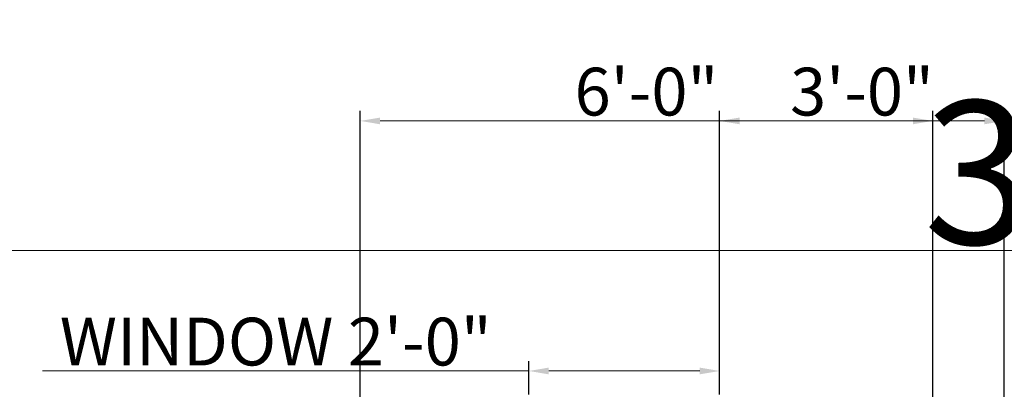
# Model space of a CAD drawing. Units: inches. Extents: x 2696 to 3240, y 1564 to 2310.
# Tile 63 of 76: x 2842 to 2966, y 2264 to 2310. Entities that reach past the tile are written whole.
import ezdxf

# ---------------------------------------------------------------- set-up
doc = ezdxf.new("R2010")
doc.units = ezdxf.units.IN
doc.layers.add('A-ANNO-DIMS', color=3, linetype='Continuous', lineweight=18)
doc.styles.add('TIMES NEW', font='times.ttf')
doc.dimstyles.new('Siddhuu', dxfattribs={"dimtxt": 6, "dimasz": 2.5, "dimexe": 1.25, "dimexo": 0.625, "dimtad": 1, "dimdec": 1, "dimlunit": 4, "dimtxsty": 'TIMES NEW', "dimcen": 2.5, "dimclrd": 256, "dimclre": 1, "dimclrt": 7, "dimadec": 0, "dimazin": 0, "dimtfac": 1, "dimtdec": 1, "dimtmove": 0, "dimatfit": 3, "dimfxl": 1, "dimtolj": 1, "dimlwd": -1, "dimarcsym": 0})

# ---------------------------------------------------------------- blocks, each defined once
blk = doc.blocks.new('*D9')
at = {"layer": 'A-ANNO-DIMS', "color": 0, "lineweight": -2, "transparency": 16777216}
for p, q in [((2745.61, 2262.83), (2745.61, 2282.19)), ((3199.61, 2262.83), (3199.61, 2282.19))]:
    blk.add_line(p, q, dxfattribs=at)
at = {"layer": 'A-ANNO-DIMS', "color": 0, "transparency": 16777216}
blk.add_line((2757.61, 2280.94), (3187.61, 2280.94), dxfattribs=at)
for points in [[(2757.61, 2282.94), (2757.61, 2278.94), (2745.61, 2280.94)], [(3187.61, 2282.94), (3187.61, 2278.94), (3199.61, 2280.94)]]:
    blk.add_solid(points, dxfattribs=at)
at = {"layer": 'Defpoints', "color": 0, "transparency": 16777216}
for p in [(3199.61, 2280.94), (2745.61, 2262.2), (3199.61, 2262.2)]:
    blk.add_point(p, dxfattribs=at)
at = {"layer": 'A-ANNO-DIMS', "color": 0, "transparency": 16777216, "insert": (2972.61, 2290.72), "char_height": 18, "attachment_point": 5, "style": 'TIMES NEW'}
blk.add_mtext("\\A1;36'", dxfattribs=at)
blk = doc.blocks.new('*D20')
at = {"layer": 'A-ANNO-DIMS', "color": 1, "lineweight": -2, "transparency": 16777216}
for p, q in [((2905.91, 2262.83), (2905.91, 2267.05)), ((2929.91, 2262.83), (2929.91, 2267.05))]:
    blk.add_line(p, q, dxfattribs=at)
at = {"layer": 'A-ANNO-DIMS', "transparency": 16777216}
for p, q in [((2905.91, 2265.8), (2844.76, 2265.8)), ((2927.41, 2265.8), (2908.41, 2265.8))]:
    blk.add_line(p, q, dxfattribs=at)
for points in [[(2908.41, 2266.22), (2908.41, 2265.38), (2905.91, 2265.8)], [(2927.41, 2266.22), (2927.41, 2265.38), (2929.91, 2265.8)]]:
    blk.add_solid(points, dxfattribs=at)
at = {"layer": 'Defpoints', "color": 0, "transparency": 16777216}
for p in [(2905.91, 2265.8), (2905.91, 2262.2), (2929.91, 2262.2)]:
    blk.add_point(p, dxfattribs=at)
at = {"layer": 'A-ANNO-DIMS', "color": 7, "transparency": 16777216, "insert": (2874.09, 2269.49), "char_height": 6, "attachment_point": 5, "style": 'TIMES NEW'}
blk.add_mtext('\\A1;WINDOW 2\'-0"', dxfattribs=at)
blk = doc.blocks.new('*D59')
at = {"layer": 'A-ANNO-DIMS', "color": 1, "lineweight": -2, "transparency": 16777216}
for p, q in [((2884.71, 1740.83), (2884.71, 2298.45)), ((2956.71, 1740.83), (2956.71, 2298.45))]:
    blk.add_line(p, q, dxfattribs=at)
at = {"layer": 'A-ANNO-DIMS', "transparency": 16777216}
blk.add_line((2887.21, 2297.2), (2954.21, 2297.2), dxfattribs=at)
for points in [[(2887.21, 2297.62), (2887.21, 2296.78), (2884.71, 2297.2)], [(2954.21, 2297.62), (2954.21, 2296.78), (2956.71, 2297.2)]]:
    blk.add_solid(points, dxfattribs=at)
at = {"layer": 'Defpoints', "color": 0, "transparency": 16777216}
for p in [(2956.71, 2297.2), (2884.71, 1740.2), (2956.71, 1740.2)]:
    blk.add_point(p, dxfattribs=at)
at = {"layer": 'A-ANNO-DIMS', "color": 7, "transparency": 16777216, "insert": (2920.71, 2300.88), "char_height": 6, "attachment_point": 5, "style": 'TIMES NEW'}
blk.add_mtext('\\A1;6\'-0"', dxfattribs=at)
blk = doc.blocks.new('*D61')
at = {"layer": 'A-ANNO-DIMS', "color": 1, "lineweight": -2, "transparency": 16777216}
for p, q in [((2965.71, 2141.33), (2965.71, 2298.45)), ((3044.3, 2141.33), (3044.3, 2298.45))]:
    blk.add_line(p, q, dxfattribs=at)
at = {"layer": 'A-ANNO-DIMS', "transparency": 16777216}
blk.add_line((2968.21, 2297.2), (3041.8, 2297.2), dxfattribs=at)
for points in [[(2968.21, 2297.62), (2968.21, 2296.78), (2965.71, 2297.2)], [(3041.8, 2297.62), (3041.8, 2296.78), (3044.3, 2297.2)]]:
    blk.add_solid(points, dxfattribs=at)
at = {"layer": 'Defpoints', "color": 0, "transparency": 16777216}
for p in [(3044.3, 2297.2), (2965.71, 2140.7), (3044.3, 2140.7)]:
    blk.add_point(p, dxfattribs=at)
at = {"layer": 'A-ANNO-DIMS', "color": 7, "transparency": 16777216, "insert": (3005.01, 2300.96), "char_height": 6, "attachment_point": 5, "style": 'TIMES NEW'}
blk.add_mtext('\\A1;6\'-6 1/2"', dxfattribs=at)
blk = doc.blocks.new('*D63')
at = {"layer": 'A-ANNO-DIMS', "color": 1, "lineweight": -2, "transparency": 16777216}
for p, q in [((2965.71, 1989.83), (2965.71, 2298.45)), ((3069.21, 1989.83), (3069.21, 2298.45))]:
    blk.add_line(p, q, dxfattribs=at)
at = {"layer": 'A-ANNO-DIMS', "transparency": 16777216}
blk.add_line((2968.21, 2297.2), (3066.71, 2297.2), dxfattribs=at)
for points in [[(2968.21, 2297.62), (2968.21, 2296.78), (2965.71, 2297.2)], [(3066.71, 2297.62), (3066.71, 2296.78), (3069.21, 2297.2)]]:
    blk.add_solid(points, dxfattribs=at)
at = {"layer": 'Defpoints', "color": 0, "transparency": 16777216}
for p in [(3069.21, 2297.2), (2965.71, 1989.2), (3069.21, 1989.2)]:
    blk.add_point(p, dxfattribs=at)
at = {"layer": 'A-ANNO-DIMS', "color": 7, "transparency": 16777216, "insert": (3017.46, 2300.96), "char_height": 6, "attachment_point": 5, "style": 'TIMES NEW'}
blk.add_mtext('\\A1;8\'-7 1/2"', dxfattribs=at)
blk = doc.blocks.new('*D70')
at = {"layer": 'A-ANNO-DIMS', "color": 1, "lineweight": -2, "transparency": 16777216}
for p, q in [((2929.91, 2262.83), (2929.91, 2298.45)), ((2965.71, 2262.83), (2965.71, 2298.45))]:
    blk.add_line(p, q, dxfattribs=at)
at = {"layer": 'A-ANNO-DIMS', "transparency": 16777216}
blk.add_line((2932.41, 2297.2), (2963.21, 2297.2), dxfattribs=at)
for points in [[(2932.41, 2297.62), (2932.41, 2296.78), (2929.91, 2297.2)], [(2963.21, 2297.62), (2963.21, 2296.78), (2965.71, 2297.2)]]:
    blk.add_solid(points, dxfattribs=at)
at = {"layer": 'Defpoints', "color": 0, "transparency": 16777216}
for p in [(2965.71, 2297.2), (2929.91, 2262.2), (2965.71, 2262.2)]:
    blk.add_point(p, dxfattribs=at)
at = {"layer": 'A-ANNO-DIMS', "color": 7, "transparency": 16777216, "insert": (2947.81, 2300.88), "char_height": 6, "attachment_point": 5, "style": 'TIMES NEW'}
blk.add_mtext('\\A1;3\'-0"', dxfattribs=at)

msp = doc.modelspace()

# ---------------------------------------------------------------- dimensions: what is measured, and where the dimension line sits
at = {"layer": 'A-ANNO-DIMS'}
for base, p1, p2, picture, middle in [((3044.3, 2297.2), (2965.71, 2140.7), (3044.3, 2140.7), '*D61', (3005.01, 2300.96)), ((3069.21, 2297.2), (2965.71, 1989.2), (3069.21, 1989.2), '*D63', (3017.46, 2300.96)), ((2956.71, 2297.2), (2884.71, 1740.2), (2956.71, 1740.2), '*D59', (2920.71, 2300.88)), ((2965.71, 2297.2), (2929.91, 2262.2), (2965.71, 2262.2), '*D70', (2947.81, 2300.88))]:
    dim = msp.add_linear_dim(base=base, p1=p1, p2=p2, dimstyle='Siddhuu', override={"dimdec": 1, "dimlfac": 1, "dimrnd": 0, "dimzin": 1, "dimdsep": 46, "dimlunit": 4, "dimfrac": 2}, dxfattribs=at)
    dim.commit()
    dim.dimension.update_dxf_attribs({"geometry": picture, "text_midpoint": middle})
dim = msp.add_linear_dim(base=(3199.61, 2280.94), p1=(2745.61, 2262.2), p2=(3199.61, 2262.2), text="36'", dimstyle='Siddhuu', override={"dimtxt": 18, "dimasz": 12, "dimclrd": 0, "dimclre": 0, "dimclrt": 0}, dxfattribs=at)
dim.commit()
dim.dimension.update_dxf_attribs({"geometry": '*D9', "text_midpoint": (2972.61, 2290.72)})
dim = msp.add_linear_dim(base=(2905.91, 2265.8), p1=(2929.91, 2262.2), p2=(2905.91, 2262.2), angle=180, text='WINDOW <>', dimstyle='Siddhuu', override={"dimdec": 1, "dimlfac": 1, "dimrnd": 0, "dimzin": 1, "dimdsep": 46, "dimlunit": 4, "dimfrac": 2}, dxfattribs=at)
dim.commit()
dim.dimension.update_dxf_attribs({"geometry": '*D20', "text_midpoint": (2874.09, 2269.49)})

doc.saveas('drawing.dxf')
